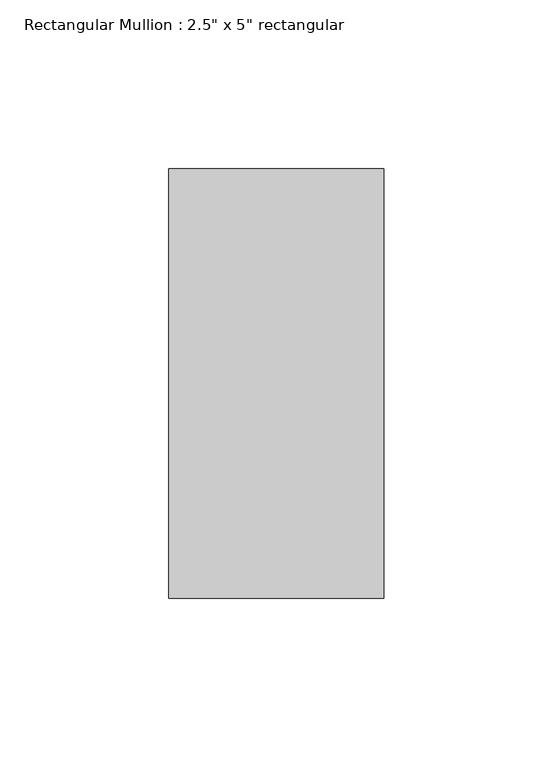
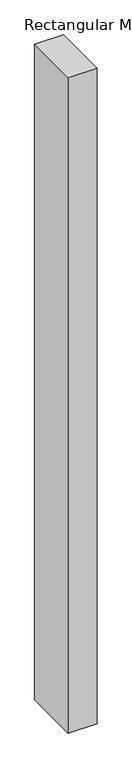
"""IFC4 building model written with IfcOpenShell, lengths in millimetres: member geometry."""

from ifc_helpers import new_model, si_unit, frame, origin, place, context, project, spatial, polyline, outline, extrude, source, transform, mapped, element, save


def member_d01054ea(model_context):
    return source(origin(), model_context, "Body", "SweptSolid", [
        extrude(outline(polyline([(31.75, 63.5), (31.75, -63.5), (-31.75, -63.5), (-31.75, 63.5), (31.75, 63.5)])), frame((0.0, 0.0, -1522.1457324), z_axis=(0.0, 0.0, 1.0), x_axis=(1.0, 0.0, 0.0)), (0.0, 0.0, 1.0), 1522.1457324),
    ])


if __name__ == "__main__":
    model = new_model("IFC4")
    model_context = context("Model", 3, world=origin())
    ifc_project = project(units=[si_unit("LENGTHUNIT", "METRE", prefix="MILLI")], contexts=[model_context])
    site = spatial("IfcSite", under=ifc_project)
    building = spatial("IfcBuilding", under=site)
    placement = place(None, origin())
    member_shape = member_d01054ea(model_context)
    element("IfcMember", 1, ObjectType="Rectangular Mullion : 2.5\" x 5\" rectangular", at=placement, inside=building, context=model_context, shape_type="MappedRepresentation", body=[
        mapped(member_shape, transform((0.0, 0.0, 0.0), x_axis=(1.0, 0.0, 0.0), y_axis=(0.0, 1.0, 0.0), z_axis=(0.0, 0.0, 1.0))),
    ])
    save(model, "model.ifc")

# Revit data of these elements
# Type "Rectangular Mullion : 2.5\" x 5\" rectangular"
#   built-in parameter 1007304 = 0.416667 (stored number, unit not read)
#   built-in parameter 1007301 = 0.104167 (stored number, unit not read)
#   built-in parameter 1007300 = 0.104167 (stored number, unit not read)
# Element 1 (IfcMember, "Rectangular Mullion : 2.5\" x 5\" rectangular")
#   Materials on its faces: "Aluminum"
# Materials
#   "Aluminum": class "Metal", colour RGB 247 247 247, transparency 0, Description = "Aluminum 6061", Cost = 0
